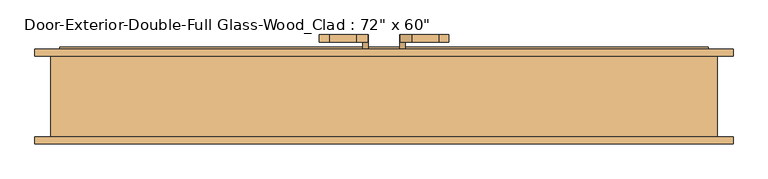
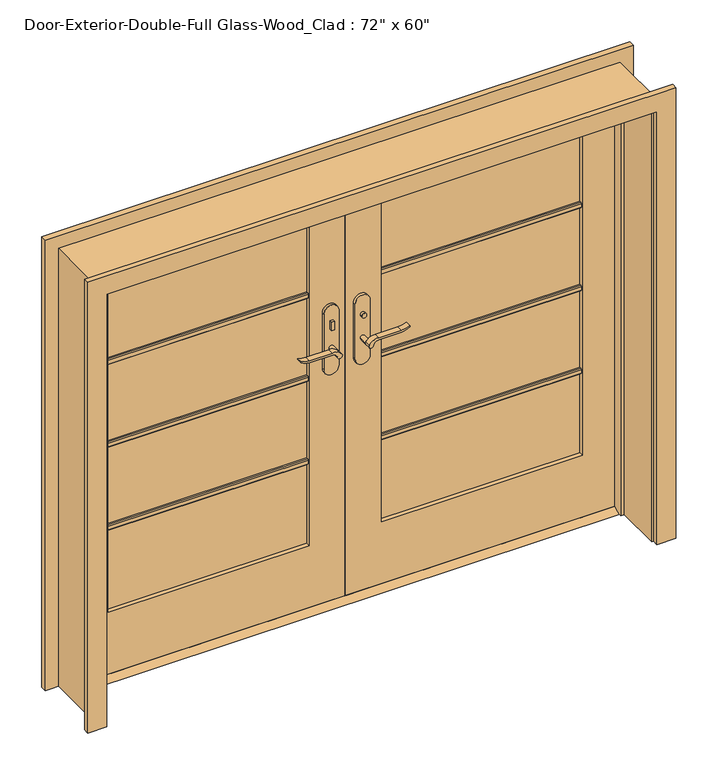
"""IFC4 building model written with IfcOpenShell, lengths in millimetres: door geometry."""

from ifc_helpers import new_model, si_unit, point, frame, frame_2d, origin, place, context, project, spatial, polyline, circle_curve, trimmed, segment, composite_curve, outline, extrude, faceted_brep, source, transform, mapped, element, save


def door_22584d03(model_context):
    return source(origin(), model_context, "Body", "SolidModel", [
        extrude(outline(polyline([(76.2, 12.7), (111.125, 12.7), (136.525, 0.0), (50.8, 0.0), (76.2, 12.7)])), frame((-914.4, 0.0, 0.0), z_axis=(1.0, 0.0, 0.0), x_axis=(0.0, 1.0, 0.0)), (0.0, 0.0, 1.0), 1828.8),
        extrude(outline(polyline([(-47.4019111, 56.2), (-57.4019111, 56.2), (-57.4019111, 66.2), (-47.4019111, 66.2), (-47.4019111, 56.2)])), frame((0.0, 0.0, 981.9), z_axis=(0.0, 0.0, 1.0), x_axis=(1.0, 0.0, 0.0)), (0.0, 0.0, 1.0), 30.0),
        extrude(outline(composite_curve([segment(trimmed(circle_curve(frame_2d((996.9, -52.4019111)), 8.0), [point((996.9, -60.4019111))], [point((996.9, -44.4019111))], False, "CARTESIAN"), True, "CONTINUOUS"), segment(trimmed(circle_curve(frame_2d((996.9, -52.4019111)), 8.0), [point((996.9, -44.4019111))], [point((996.9, -60.4019111))], False, "CARTESIAN"), True, "CONTINUOUS")], self_intersect=False)), frame((0.0, 121.125, 0.0), z_axis=(0.0, 1.0, 0.0), x_axis=(0.0, 0.0, 1.0)), (0.0, 0.0, 1.0), 10.0),
        extrude(outline(composite_curve([segment(trimmed(circle_curve(frame_2d((897.1555521, -76.0694241)), 37.2832219), [point((919.0523287, -45.8937749))], [point((934.4, -77.7693445))], False, "CARTESIAN"), True, "CONTINUOUS"), segment(polyline([(934.4, -77.7693445), (934.4, -154.045502)]), True, "CONTINUOUS"), segment(trimmed(circle_curve(frame_2d((1017.6850638, -153.9791202)), 83.2850902), [point((934.4, -154.045502))], [point((939.4, -182.4019111))], True, "CARTESIAN"), True, "CONTINUOUS"), segment(polyline([(939.4, -182.4019111), (936.6135558, -182.4019111)]), True, "CONTINUOUS"), segment(trimmed(circle_curve(frame_2d((986.6709207, -150.4622499)), 59.3791355), [point((936.6135558, -182.4019111))], [point((927.4, -154.045502))], False, "CARTESIAN"), True, "CONTINUOUS"), segment(polyline([(927.4, -154.045502), (927.4, -77.7881013)]), True, "CONTINUOUS"), segment(trimmed(circle_curve(frame_2d((909.2738613, -77.7881013)), 18.1261387), [point((927.4, -77.7881013))], [point((914.4, -60.4019111))], True, "CARTESIAN"), True, "CONTINUOUS"), segment(trimmed(circle_curve(frame_2d((914.4, -52.4019111)), 8.0), [point((914.4, -60.4019111))], [point((919.0523287, -45.8937749))], False, "CARTESIAN"), True, "CONTINUOUS")], self_intersect=False)), frame((0.0, 16.2, 0.0), z_axis=(0.0, 1.0, 0.0), x_axis=(0.0, 0.0, 1.0)), (0.0, 0.0, 1.0), 20.0),
        extrude(outline(composite_curve([segment(trimmed(circle_curve(frame_2d((914.4, -52.4019111)), 8.0), [point((914.3999903, -60.4019111))], [point((919.0523287, -45.8937749))], False, "CARTESIAN"), True, "CONTINUOUS"), segment(trimmed(circle_curve(frame_2d((897.1555521, -76.0694241)), 37.2832219), [point((919.0523287, -45.8937749))], [point((934.4, -77.7693445))], False, "CARTESIAN"), True, "CONTINUOUS"), segment(polyline([(934.4, -77.7693445), (934.4, -154.045502)]), True, "CONTINUOUS"), segment(trimmed(circle_curve(frame_2d((1017.6850638, -153.9791202)), 83.2850902), [point((934.4, -154.045502))], [point((939.4, -182.4019111))], True, "CARTESIAN"), True, "CONTINUOUS"), segment(polyline([(939.4, -182.4019111), (936.6135558, -182.4019111)]), True, "CONTINUOUS"), segment(trimmed(circle_curve(frame_2d((986.6709207, -150.4622499)), 59.3791355), [point((936.6135558, -182.4019111))], [point((927.4, -154.045502))], False, "CARTESIAN"), True, "CONTINUOUS"), segment(polyline([(927.4, -154.045502), (927.4, -77.788099)]), True, "CONTINUOUS"), segment(trimmed(circle_curve(frame_2d((909.2738682, -77.788099)), 18.1261318), [point((927.4, -77.788099))], [point((914.3999903, -60.4019111))], True, "CARTESIAN"), True, "CONTINUOUS")], self_intersect=False)), frame((0.0, 151.125, 0.0), z_axis=(0.0, 1.0, 0.0), x_axis=(0.0, 0.0, 1.0)), (0.0, 0.0, 1.0), 20.0),
        extrude(outline(composite_curve([segment(trimmed(circle_curve(frame_2d((914.4, -52.4019111)), 8.0), [point((914.4, -60.4019111))], [point((914.4, -44.4019111))], False, "CARTESIAN"), True, "CONTINUOUS"), segment(trimmed(circle_curve(frame_2d((914.4, -52.4019111)), 8.0), [point((914.4, -44.4019111))], [point((914.4, -60.4019111))], False, "CARTESIAN"), True, "CONTINUOUS")], self_intersect=False)), frame((0.0, 36.2, 0.0), z_axis=(0.0, 1.0, 0.0), x_axis=(0.0, 0.0, 1.0)), (0.0, 0.0, 1.0), 30.0),
        extrude(outline(composite_curve([segment(trimmed(circle_curve(frame_2d((914.4, -52.4019111)), 8.0), [point((914.4, -60.4019111))], [point((914.4, -44.4019111))], False, "CARTESIAN"), True, "CONTINUOUS"), segment(trimmed(circle_curve(frame_2d((914.4, -52.4019111)), 8.0), [point((914.4, -44.4019111))], [point((914.4, -60.4019111))], False, "CARTESIAN"), True, "CONTINUOUS")], self_intersect=False)), frame((0.0, 121.125, 0.0), z_axis=(0.0, 1.0, 0.0), x_axis=(0.0, 0.0, 1.0)), (0.0, 0.0, 1.0), 30.0),
        extrude(outline(composite_curve([segment(polyline([(844.4, -27.4019111), (1039.4, -27.4019111)]), True, "CONTINUOUS"), segment(trimmed(circle_curve(frame_2d((1039.4, -52.4019111)), 25.0), [point((1039.4, -27.4019111))], [point((1039.4, -77.4019111))], False, "CARTESIAN"), True, "CONTINUOUS"), segment(polyline([(1039.4, -77.4019111), (844.4, -77.4019111)]), True, "CONTINUOUS"), segment(trimmed(circle_curve(frame_2d((844.4, -52.4019111)), 25.0), [point((844.4, -77.4019111))], [point((844.4, -27.4019111))], False, "CARTESIAN"), True, "CONTINUOUS")], self_intersect=False)), frame((0.0, 66.2, 0.0), z_axis=(0.0, 1.0, 0.0), x_axis=(0.0, 0.0, 1.0)), (0.0, 0.0, 1.0), 10.0),
        extrude(outline(composite_curve([segment(polyline([(844.4, -27.4019111), (1039.4, -27.4019111)]), True, "CONTINUOUS"), segment(trimmed(circle_curve(frame_2d((1039.4, -52.4019111)), 25.0), [point((1039.4, -27.4019111))], [point((1039.4, -77.4019111))], False, "CARTESIAN"), True, "CONTINUOUS"), segment(polyline([(1039.4, -77.4019111), (844.4, -77.4019111)]), True, "CONTINUOUS"), segment(trimmed(circle_curve(frame_2d((844.4, -52.4019111)), 25.0), [point((844.4, -77.4019111))], [point((844.4, -27.4019111))], False, "CARTESIAN"), True, "CONTINUOUS")], self_intersect=False)), frame((0.0, 111.125, 0.0), z_axis=(0.0, 1.0, 0.0), x_axis=(0.0, 0.0, 1.0)), (0.0, 0.0, 1.0), 10.0),
        extrude(outline(polyline([(47.3875, 131.125), (57.3875, 131.125), (57.3875, 121.125), (47.3875, 121.125), (47.3875, 131.125)])), frame((0.0, 0.0, 981.9), z_axis=(0.0, 0.0, 1.0), x_axis=(1.0, 0.0, 0.0)), (0.0, 0.0, 1.0), 30.0),
        extrude(outline(composite_curve([segment(trimmed(circle_curve(frame_2d((996.9, 52.3875)), 8.0), [point((996.9, 60.3875))], [point((996.9, 44.3875))], False, "CARTESIAN"), True, "CONTINUOUS"), segment(trimmed(circle_curve(frame_2d((996.9, 52.3875)), 8.0), [point((996.9, 44.3875))], [point((996.9, 60.3875))], False, "CARTESIAN"), True, "CONTINUOUS")], self_intersect=False)), frame((0.0, 56.2, 0.0), z_axis=(0.0, 1.0, 0.0), x_axis=(0.0, 0.0, 1.0)), (0.0, 0.0, 1.0), 10.0),
        extrude(outline(composite_curve([segment(trimmed(circle_curve(frame_2d((914.4, 52.3875)), 8.0), [point((919.0523287, 45.8793637))], [point((914.4, 60.3875))], False, "CARTESIAN"), True, "CONTINUOUS"), segment(trimmed(circle_curve(frame_2d((909.2738613, 77.7736901)), 18.1261387), [point((914.4, 60.3875))], [point((927.4, 77.7736901))], True, "CARTESIAN"), True, "CONTINUOUS"), segment(polyline([(927.4, 77.7736901), (927.4, 154.0310909)]), True, "CONTINUOUS"), segment(trimmed(circle_curve(frame_2d((986.6709207, 150.4478388)), 59.3791355), [point((927.4, 154.0310909))], [point((936.6135558, 182.3875))], False, "CARTESIAN"), True, "CONTINUOUS"), segment(polyline([(936.6135558, 182.3875), (939.4, 182.3875)]), True, "CONTINUOUS"), segment(trimmed(circle_curve(frame_2d((1017.6850638, 153.9647091)), 83.2850902), [point((939.4, 182.3875))], [point((934.4, 154.0310909))], True, "CARTESIAN"), True, "CONTINUOUS"), segment(polyline([(934.4, 154.0310909), (934.4, 77.7549333)]), True, "CONTINUOUS"), segment(trimmed(circle_curve(frame_2d((897.1555521, 76.0550129)), 37.2832219), [point((934.4, 77.7549333))], [point((919.0523287, 45.8793637))], False, "CARTESIAN"), True, "CONTINUOUS")], self_intersect=False)), frame((0.0, 151.125, 0.0), z_axis=(0.0, 1.0, 0.0), x_axis=(0.0, 0.0, 1.0)), (0.0, 0.0, 1.0), 20.0),
        extrude(outline(composite_curve([segment(trimmed(circle_curve(frame_2d((909.2738682, 77.7736878)), 18.1261318), [point((914.3999903, 60.3875))], [point((927.4, 77.7736878))], True, "CARTESIAN"), True, "CONTINUOUS"), segment(polyline([(927.4, 77.7736878), (927.4, 154.0310909)]), True, "CONTINUOUS"), segment(trimmed(circle_curve(frame_2d((986.6709207, 150.4478388)), 59.3791355), [point((927.4, 154.0310909))], [point((936.6135558, 182.3875))], False, "CARTESIAN"), True, "CONTINUOUS"), segment(polyline([(936.6135558, 182.3875), (939.4, 182.3875)]), True, "CONTINUOUS"), segment(trimmed(circle_curve(frame_2d((1017.6850638, 153.9647091)), 83.2850902), [point((939.4, 182.3875))], [point((934.4, 154.0310909))], True, "CARTESIAN"), True, "CONTINUOUS"), segment(polyline([(934.4, 154.0310909), (934.4, 77.7549333)]), True, "CONTINUOUS"), segment(trimmed(circle_curve(frame_2d((897.1555521, 76.0550129)), 37.2832219), [point((934.4, 77.7549333))], [point((919.0523287, 45.8793637))], False, "CARTESIAN"), True, "CONTINUOUS"), segment(trimmed(circle_curve(frame_2d((914.4, 52.3875)), 8.0), [point((919.0523287, 45.8793637))], [point((914.3999903, 60.3875))], False, "CARTESIAN"), True, "CONTINUOUS")], self_intersect=False)), frame((0.0, 16.2, 0.0), z_axis=(0.0, 1.0, 0.0), x_axis=(0.0, 0.0, 1.0)), (0.0, 0.0, 1.0), 20.0),
        extrude(outline(composite_curve([segment(trimmed(circle_curve(frame_2d((914.4, 52.3875)), 8.0), [point((914.4, 60.3875))], [point((914.4, 44.3875))], False, "CARTESIAN"), True, "CONTINUOUS"), segment(trimmed(circle_curve(frame_2d((914.4, 52.3875)), 8.0), [point((914.4, 44.3875))], [point((914.4, 60.3875))], False, "CARTESIAN"), True, "CONTINUOUS")], self_intersect=False)), frame((0.0, 121.125, 0.0), z_axis=(0.0, 1.0, 0.0), x_axis=(0.0, 0.0, 1.0)), (0.0, 0.0, 1.0), 30.0),
        extrude(outline(composite_curve([segment(trimmed(circle_curve(frame_2d((914.4, 52.3875)), 8.0), [point((914.4, 60.3875))], [point((914.4, 44.3875))], False, "CARTESIAN"), True, "CONTINUOUS"), segment(trimmed(circle_curve(frame_2d((914.4, 52.3875)), 8.0), [point((914.4, 44.3875))], [point((914.4, 60.3875))], False, "CARTESIAN"), True, "CONTINUOUS")], self_intersect=False)), frame((0.0, 36.2, 0.0), z_axis=(0.0, 1.0, 0.0), x_axis=(0.0, 0.0, 1.0)), (0.0, 0.0, 1.0), 30.0),
        extrude(outline(composite_curve([segment(trimmed(circle_curve(frame_2d((844.4, 52.3875)), 25.0), [point((844.4, 27.3875))], [point((844.4, 77.3875))], False, "CARTESIAN"), True, "CONTINUOUS"), segment(polyline([(844.4, 77.3875), (1039.4, 77.3875)]), True, "CONTINUOUS"), segment(trimmed(circle_curve(frame_2d((1039.4, 52.3875)), 25.0), [point((1039.4, 77.3875))], [point((1039.4, 27.3875))], False, "CARTESIAN"), True, "CONTINUOUS"), segment(polyline([(1039.4, 27.3875), (844.4, 27.3875)]), True, "CONTINUOUS")], self_intersect=False)), frame((0.0, 111.125, 0.0), z_axis=(0.0, 1.0, 0.0), x_axis=(0.0, 0.0, 1.0)), (0.0, 0.0, 1.0), 10.0),
        extrude(outline(composite_curve([segment(trimmed(circle_curve(frame_2d((844.4, 52.3875)), 25.0), [point((844.4, 27.3875))], [point((844.4, 77.3875))], False, "CARTESIAN"), True, "CONTINUOUS"), segment(polyline([(844.4, 77.3875), (1039.4, 77.3875)]), True, "CONTINUOUS"), segment(trimmed(circle_curve(frame_2d((1039.4, 52.3875)), 25.0), [point((1039.4, 77.3875))], [point((1039.4, 27.3875))], False, "CARTESIAN"), True, "CONTINUOUS"), segment(polyline([(1039.4, 27.3875), (844.4, 27.3875)]), True, "CONTINUOUS")], self_intersect=False)), frame((0.0, 66.2, 0.0), z_axis=(0.0, 1.0, 0.0), x_axis=(0.0, 0.0, 1.0)), (0.0, 0.0, 1.0), 10.0),
        extrude(outline(polyline([(90.17, 1121.171875), (90.17, 1102.121875), (83.82, 1102.121875), (80.645, 1105.296875), (80.645, 1117.996875), (83.82, 1121.171875), (90.17, 1121.171875)])), frame((120.65, 0.0, 0.0), z_axis=(1.0, 0.0, 0.0), x_axis=(0.0, 1.0, 0.0)), (0.0, 0.0, 1.0), 673.1),
        extrude(outline(polyline([(90.17, 827.88125), (90.17, 808.83125), (83.82, 808.83125), (80.645, 812.00625), (80.645, 824.70625), (83.82, 827.88125), (90.17, 827.88125)])), frame((120.65, 0.0, 0.0), z_axis=(1.0, 0.0, 0.0), x_axis=(0.0, 1.0, 0.0)), (0.0, 0.0, 1.0), 673.1),
        extrude(outline(polyline([(90.17, 534.590625), (90.17, 515.540625), (83.82, 515.540625), (80.645, 518.715625), (80.645, 531.415625), (83.82, 534.590625), (90.17, 534.590625)])), frame((120.65, 0.0, 0.0), z_axis=(1.0, 0.0, 0.0), x_axis=(0.0, 1.0, 0.0)), (0.0, 0.0, 1.0), 673.1),
        extrude(outline(polyline([(97.155, 1121.171875), (103.505, 1121.171875), (106.68, 1117.996875), (106.68, 1105.296875), (103.505, 1102.121875), (97.155, 1102.121875), (97.155, 1121.171875)])), frame((-793.75, 0.0, 0.0), z_axis=(1.0, 0.0, 0.0), x_axis=(0.0, 1.0, 0.0)), (0.0, 0.0, 1.0), 673.1),
        extrude(outline(polyline([(97.155, 827.88125), (103.505, 827.88125), (106.68, 824.70625), (106.68, 812.00625), (103.505, 808.83125), (97.155, 808.83125), (97.155, 827.88125)])), frame((-793.75, 0.0, 0.0), z_axis=(1.0, 0.0, 0.0), x_axis=(0.0, 1.0, 0.0)), (0.0, 0.0, 1.0), 673.1),
        extrude(outline(polyline([(97.155, 534.590625), (103.505, 534.590625), (106.68, 531.415625), (106.68, 518.715625), (103.505, 515.540625), (97.155, 515.540625), (97.155, 534.590625)])), frame((-793.75, 0.0, 0.0), z_axis=(1.0, 0.0, 0.0), x_axis=(0.0, 1.0, 0.0)), (0.0, 0.0, 1.0), 673.1),
        extrude(outline(polyline([(97.155, 1121.171875), (103.505, 1121.171875), (106.68, 1117.996875), (106.68, 1105.296875), (103.505, 1102.121875), (97.155, 1102.121875), (97.155, 1121.171875)])), frame((120.65, 0.0, 0.0), z_axis=(1.0, 0.0, 0.0), x_axis=(0.0, 1.0, 0.0)), (0.0, 0.0, 1.0), 673.1),
        extrude(outline(polyline([(97.155, 827.88125), (103.505, 827.88125), (106.68, 824.70625), (106.68, 812.00625), (103.505, 808.83125), (97.155, 808.83125), (97.155, 827.88125)])), frame((120.65, 0.0, 0.0), z_axis=(1.0, 0.0, 0.0), x_axis=(0.0, 1.0, 0.0)), (0.0, 0.0, 1.0), 673.1),
        extrude(outline(polyline([(97.155, 534.590625), (103.505, 534.590625), (106.68, 531.415625), (106.68, 518.715625), (103.505, 515.540625), (97.155, 515.540625), (97.155, 534.590625)])), frame((120.65, 0.0, 0.0), z_axis=(1.0, 0.0, 0.0), x_axis=(0.0, 1.0, 0.0)), (0.0, 0.0, 1.0), 673.1),
        extrude(outline(polyline([(90.17, 1121.171875), (90.17, 1102.121875), (83.82, 1102.121875), (80.645, 1105.296875), (80.645, 1117.996875), (83.82, 1121.171875), (90.17, 1121.171875)])), frame((-793.75, 0.0, 0.0), z_axis=(1.0, 0.0, 0.0), x_axis=(0.0, 1.0, 0.0)), (0.0, 0.0, 1.0), 673.1),
        extrude(outline(polyline([(90.17, 827.88125), (90.17, 808.83125), (83.82, 808.83125), (80.645, 812.00625), (80.645, 824.70625), (83.82, 827.88125), (90.17, 827.88125)])), frame((-793.75, 0.0, 0.0), z_axis=(1.0, 0.0, 0.0), x_axis=(0.0, 1.0, 0.0)), (0.0, 0.0, 1.0), 673.1),
        extrude(outline(polyline([(90.17, 534.590625), (90.17, 515.540625), (83.82, 515.540625), (80.645, 518.715625), (80.645, 531.415625), (83.82, 534.590625), (90.17, 534.590625)])), frame((-793.75, 0.0, 0.0), z_axis=(1.0, 0.0, 0.0), x_axis=(0.0, 1.0, 0.0)), (0.0, 0.0, 1.0), 673.1),
        extrude(outline(polyline([(0.0, 920.75), (0.0, 984.25), (1593.85, 984.25), (1593.85, -984.25), (0.0, -984.25), (0.0, -920.75), (1530.35, -920.75), (1530.35, 920.75), (0.0, 920.75)])), frame((0.0, 111.125, 0.0), z_axis=(0.0, 1.0, 0.0), x_axis=(0.0, 0.0, 1.0)), (0.0, 0.0, 1.0), 19.05),
        extrude(outline(polyline([(0.0, 920.75), (0.0, 984.25), (1593.85, 984.25), (1593.85, -984.25), (0.0, -984.25), (0.0, -920.75), (1530.35, -920.75), (1530.35, 920.75), (0.0, 920.75)])), frame((0.0, -136.525, 0.0), z_axis=(0.0, 1.0, 0.0), x_axis=(0.0, 0.0, 1.0)), (0.0, 0.0, 1.0), 19.05),
        extrude(outline(polyline([(12.7, 914.4), (1524.0, 914.4), (1524.0, 1.5875), (12.7, 1.5875), (12.7, 914.4)]), holes=[polyline([(1404.9375, 120.65), (1404.9375, 793.75), (231.775, 793.75), (231.775, 120.65), (1404.9375, 120.65)])]), frame((0.0, 76.2, 0.0), z_axis=(0.0, 1.0, 0.0), x_axis=(0.0, 0.0, 1.0)), (0.0, 0.0, 1.0), 34.925),
        extrude(outline(polyline([(1524.0, -914.4), (12.7, -914.4), (12.7, -1.6019111), (1524.0, -1.6019111), (1524.0, -914.4)]), holes=[polyline([(231.775, -793.75), (1404.9375, -793.75), (1404.9375, -120.65), (231.775, -120.65), (231.775, -793.75)])]), frame((0.0, 76.2, 0.0), z_axis=(0.0, 1.0, 0.0), x_axis=(0.0, 0.0, 1.0)), (0.0, 0.0, 1.0), 34.925),
        faceted_brep([(939.8, 111.125, 0.0), (939.8, -117.475, 0.0), (914.4, -117.475, 0.0), (914.4, 41.275, 0.0), (901.7, 41.275, 0.0), (901.7, 76.2, 0.0), (914.4, 76.2, 0.0), (914.4, 111.125, 0.0), (939.8, 111.125, 1549.4), (939.8, -117.475, 1549.4), (-939.8, -117.475, 1549.4), (-939.8, -117.475, 0.0), (-914.4, -117.475, 0.0), (-914.4, -117.475, 1524.0), (914.4, -117.475, 1524.0), (914.4, 41.275, 1524.0), (-914.4, 41.275, 1524.0), (-914.4, 41.275, 0.0), (-901.7, 41.275, 0.0), (-901.7, 41.275, 1511.3), (901.7, 41.275, 1511.3), (901.7, 76.2, 1511.3), (1.5875, 76.2, 1511.3), (-1.6019111, 76.2, 1511.3), (-901.7, 76.2, 1511.3), (-901.7, 76.2, 0.0), (-914.4, 76.2, 0.0), (-914.4, 76.2, 1524.0), (-1.6019111, 76.2, 1524.0), (1.5875, 76.2, 1524.0), (914.4, 76.2, 1524.0), (914.4, 111.125, 1524.0), (1.5875, 111.125, 1524.0), (-1.6019111, 111.125, 1524.0), (-914.4, 111.125, 1524.0), (-914.4, 111.125, 0.0), (-939.8, 111.125, 0.0), (-939.8, 111.125, 1549.4)], [[[0, 1, 2, 3, 4, 5, 6, 7]], [[1, 0, 8, 9]], [[2, 1, 9, 10, 11, 12, 13, 14]], [[3, 2, 14, 15]], [[4, 3, 15, 16, 17, 18, 19, 20]], [[5, 4, 20, 21]], [[6, 5, 21, 22, 23, 24, 25, 26, 27, 28, 29, 30]], [[7, 6, 30, 31]], [[0, 7, 31, 32, 33, 34, 35, 36, 37, 8]], [[9, 8, 37, 10]], [[14, 13, 16, 15]], [[20, 19, 24, 23, 22, 21]], [[31, 30, 29, 28, 27, 34, 33, 32]], [[12, 11, 36, 35, 26, 25, 18, 17]], [[11, 10, 37, 36]], [[13, 12, 17, 16]], [[19, 18, 25, 24]], [[27, 26, 35, 34]]]),
        extrude(outline(polyline([(793.75, 90.17), (120.65, 90.17), (120.65, 97.155), (793.75, 97.155), (793.75, 90.17)])), frame((0.0, 0.0, 231.775), z_axis=(0.0, 0.0, 1.0), x_axis=(1.0, 0.0, 0.0)), (0.0, 0.0, 1.0), 1173.1625),
        extrude(outline(polyline([(-120.65, 90.17), (-793.75, 90.17), (-793.75, 97.155), (-120.65, 97.155), (-120.65, 90.17)])), frame((0.0, 0.0, 231.775), z_axis=(0.0, 0.0, 1.0), x_axis=(1.0, 0.0, 0.0)), (0.0, 0.0, 1.0), 1173.1625),
    ])


if __name__ == "__main__":
    model = new_model("IFC4")
    model_context = context("Model", 3, world=origin())
    ifc_project = project(units=[si_unit("LENGTHUNIT", "METRE", prefix="MILLI")], contexts=[model_context])
    site = spatial("IfcSite", under=ifc_project)
    building = spatial("IfcBuilding", under=site)
    placement = place(None, origin())
    door_shape = door_22584d03(model_context)
    element("IfcDoor", 1, ObjectType="Door-Exterior-Double-Full Glass-Wood_Clad : 72\" x 60\"", at=placement, inside=building, context=model_context, shape_type="MappedRepresentation", body=[
        mapped(door_shape, transform((0.0, 0.0, 0.0), x_axis=(1.0, 0.0, 0.0), y_axis=(0.0, 1.0, 0.0), z_axis=(0.0, 0.0, 1.0))),
    ])
    save(model, "model.ifc")

# Revit data of these elements
# Type "Door-Exterior-Double-Full Glass-Wood_Clad : 72\" x 60\""
#   Type Mark = "9"
#   Assembly Code = "B2030100"
#   Analytic Construction = "French door, wood frame with double glass"
#   Top Rail = 0' - 4 11/16"
#   Threshold Offset [instance default] = 0' - 0 1/2"
#   Thickness = 0' - 1 3/8"
#   Thermal Resistance (R) = 1.9158 (h·ft²·°F)/BTU
#   Swing Angle [instance default] = 90.00°
#   Stiles = 0' - 4 3/4"
#   Rough Width = 6' - 2"
#   Rough Height = 5' - 1"
#   Panel Width = 3' - 0"
#   Door Offset [instance default] = 0' - 0"
#   Height = 5' - 0"
#   Width = 6' - 0"
#   Heat Transfer Coefficient (U) = 0.5220 BTU/(h·ft²·°F)
#   Bottom Rail = 0' - 9 1/8"
#   Exterior Trim [instance default] = yes
#   Threshold [instance default] = yes
#   Show Grill [instance default] = yes
#   Function = 1
#   Trim Material = Cherry
#   Threshold Material = Cherry
#   Panel Material = Cherry
#   Glazing = Glass
#   Frame Material = Cherry
#   Door Handle Material = Aluminum
#   Visual Light Transmittance = 0
#   Solar Heat Gain Coefficient = 0
#   Wall Closure = (empty or 0)
#   Construction Type = (empty or 0)
# Element 1 (IfcDoor, "Door-Exterior-Double-Full Glass-Wood_Clad : 72\" x 60\"")
#   Materials on its faces: "Cherry", "Aluminum", "Glass"
# Materials
#   "Cherry": class "Wood", colour RGB 226 177 128, transparency 0, Description = "Prunus Serotina", Cost = 0
#   "Glass": class "Glass", colour RGB 0 128 192, transparency 0.75, Description = "Soda Lime Glass", Cost = 0
#   "Aluminum": class "Metal", colour RGB 247 247 247, transparency 0, Description = "Aluminum 6061", Cost = 0
